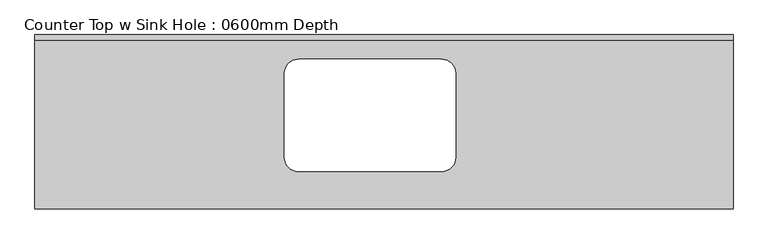
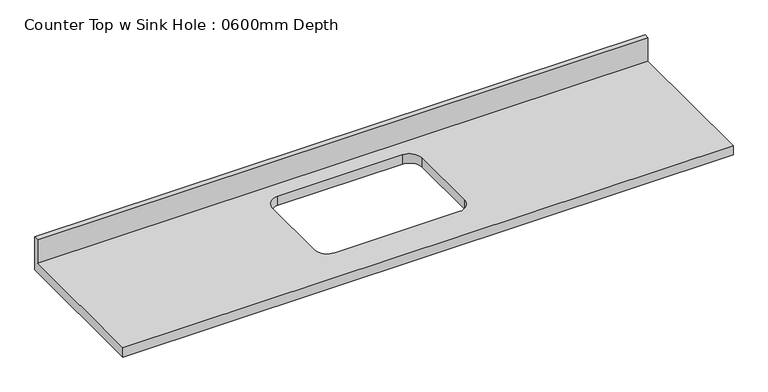
"""IFC4 building model written with IfcOpenShell, lengths in millimetres: furniture geometry, Counter Top w Sink Hole : 0600mm Depth."""

from ifc_helpers import new_model, si_unit, frame, origin, place, context, project, spatial, polyline, circle_curve, source, transform, mapped, element, save
from ifc_brep_helpers import plane_surface, revolved_surface, advanced_brep


def counter_top_w_sink_hole_0600mm_depth_f226a61d(model_context):
    return source(origin(), model_context, "Body", "AdvancedBrep", [
        advanced_brep(
        [(-1200.4622951, -624.68125, 900.1125), (1299.8502049, -624.68125, 900.1125), (1299.8502049, -19.05, 900.1125), (-1200.4622951, -19.05, 900.1125), (-255.8997951, -87.3125, 900.1125), (255.2752049, -87.3125, 900.1125), (306.0752049, -138.1125, 900.1125), (306.0752049, -439.7375, 900.1125), (255.2752049, -490.5375, 900.1125), (-255.8997951, -490.5375, 900.1125), (-306.6997951, -439.7375, 900.1125), (-306.6997951, -138.1125, 900.1125), (1299.8502049, 0.0, 860.425), (1299.8502049, -624.68125, 860.425), (-1200.4622951, -624.68125, 860.425), (-1200.4622951, 0.0, 860.425), (255.2752049, -87.3125, 860.425), (-255.8997951, -87.3125, 860.425), (-306.6997951, -138.1125, 860.425), (-306.6997951, -439.7375, 860.425), (-255.8997951, -490.5375, 860.425), (255.2752049, -490.5375, 860.425), (306.0752049, -439.7375, 860.425), (306.0752049, -138.1125, 860.425), (-1200.4622951, 0.0, 1001.7125), (1299.8502049, 0.0, 1001.7125), (-1200.4622951, -19.05, 1001.7125), (1299.8502049, -19.05, 1001.7125)],
        [
            (0, 1),
            (1, 2),
            (2, 3),
            (3, 0),
            (4, 5),
            (5, 6, circle_curve(frame((255.2752049, -138.1125, 900.1125), z_axis=(0.0, 0.0, -1.0), x_axis=(1.0, 0.0, 0.0)), 50.8)),
            (6, 7),
            (7, 8, circle_curve(frame((255.2752049, -439.7375, 900.1125), z_axis=(0.0, 0.0, -1.0), x_axis=(1.0, 0.0, 0.0)), 50.8)),
            (8, 9),
            (9, 10, circle_curve(frame((-255.8997951, -439.7375, 900.1125), z_axis=(0.0, 0.0, -1.0), x_axis=(1.0, 0.0, 0.0)), 50.8)),
            (10, 11),
            (11, 4, circle_curve(frame((-255.8997951, -138.1125, 900.1125), z_axis=(0.0, 0.0, -1.0), x_axis=(1.0, 0.0, 0.0)), 50.8)),
            (12, 13),
            (13, 14),
            (14, 15),
            (15, 12),
            (16, 17),
            (17, 18, circle_curve(frame((-255.8997951, -138.1125, 860.425), z_axis=(0.0, 0.0, 1.0), x_axis=(1.0, 0.0, 0.0)), 50.8)),
            (18, 19),
            (19, 20, circle_curve(frame((-255.8997951, -439.7375, 860.425), z_axis=(0.0, 0.0, 1.0), x_axis=(1.0, 0.0, 0.0)), 50.8)),
            (20, 21),
            (21, 22, circle_curve(frame((255.2752049, -439.7375, 860.425), z_axis=(0.0, 0.0, 1.0), x_axis=(1.0, 0.0, 0.0)), 50.8)),
            (22, 23),
            (23, 16, circle_curve(frame((255.2752049, -138.1125, 860.425), z_axis=(0.0, 0.0, 1.0), x_axis=(1.0, 0.0, 0.0)), 50.8)),
            (15, 24),
            (24, 25),
            (25, 12),
            (14, 0),
            (3, 26),
            (26, 24),
            (13, 1),
            (25, 27),
            (27, 2),
            (26, 27),
            (4, 17),
            (16, 5),
            (11, 18),
            (10, 19),
            (9, 20),
            (8, 21),
            (7, 22),
            (6, 23),
        ],
        [
            plane_surface(frame((-1200.4622951, 0.0, 900.1125), z_axis=(0.0, 0.0, 1.0), x_axis=(-1.0, 0.0, 0.0))),
            plane_surface(frame((-1200.4622951, 0.0, 860.425), z_axis=(0.0, 0.0, -1.0), x_axis=(1.0, 0.0, 0.0))),
            plane_surface(frame((1299.8502049, 0.0, 900.1125), z_axis=(0.0, 1.0, 0.0), x_axis=(0.0, 0.0, -1.0))),
            plane_surface(frame((-1200.4622951, 0.0, 900.1125), z_axis=(-1.0, 0.0, 0.0), x_axis=(0.0, 0.0, -1.0))),
            plane_surface(frame((-1200.4622951, -624.68125, 900.1125), z_axis=(0.0, -1.0, 0.0), x_axis=(0.0, 0.0, -1.0))),
            plane_surface(frame((1299.8502049, -624.68125, 900.1125), z_axis=(1.0, 0.0, 0.0), x_axis=(0.0, 0.0, -1.0))),
            plane_surface(frame((-1200.4622951, 0.0, 1001.7125), z_axis=(0.0, 0.0, 1.0), x_axis=(0.0, -1.0, 0.0))),
            plane_surface(frame((-1200.4622951, -19.05, 1001.7125), z_axis=(0.0, -1.0, 0.0), x_axis=(0.0, 0.0, -1.0))),
            plane_surface(frame((255.2752049, -87.3125, 900.1125), z_axis=(0.0, -1.0, 0.0), x_axis=(0.0, 0.0, -1.0))),
            revolved_surface(polyline([(-205.0997951, -138.1125, 900.1125), (-205.0997951, -138.1125, 860.425)]), (-255.8997951, -138.1125, 860.425), (0.0, 0.0, 1.0)),
            plane_surface(frame((-306.6997951, -138.1125, 900.1125), z_axis=(1.0, 0.0, 0.0), x_axis=(0.0, 0.0, -1.0))),
            revolved_surface(polyline([(-205.0997951, -439.7375, 900.1125), (-205.0997951, -439.7375, 860.425)]), (-255.8997951, -439.7375, 860.425), (0.0, 0.0, 1.0)),
            plane_surface(frame((-255.8997951, -490.5375, 900.1125), z_axis=(0.0, 1.0, 0.0), x_axis=(0.0, 0.0, -1.0))),
            revolved_surface(polyline([(306.0752049, -439.7375, 900.1125), (306.0752049, -439.7375, 860.425)]), (255.2752049, -439.7375, 860.425), (0.0, 0.0, 1.0)),
            plane_surface(frame((306.0752049, -439.7375, 900.1125), z_axis=(-1.0, 0.0, 0.0), x_axis=(0.0, 0.0, -1.0))),
            revolved_surface(polyline([(306.0752049, -138.1125, 900.1125), (306.0752049, -138.1125, 860.425)]), (255.2752049, -138.1125, 860.425), (0.0, 0.0, 1.0)),
        ],
        [
            (0, [[1, 2, 3, 4], [5, 6, 7, 8, 9, 10, 11, 12]]),
            (1, [[13, 14, 15, 16], [17, 18, 19, 20, 21, 22, 23, 24]]),
            (2, [[-16, 25, 26, 27]]),
            (3, [[-15, 28, -4, 29, 30, -25]]),
            (4, [[-1, -28, -14, 31]]),
            (5, [[-13, -27, 32, 33, -2, -31]]),
            (6, [[-30, 34, -32, -26]]),
            (7, [[-34, -29, -3, -33]]),
            (8, [[35, -17, 36, -5]]),
            (9, [[-35, -12, 37, -18]]),
            (10, [[-37, -11, 38, -19]]),
            (11, [[-38, -10, 39, -20]]),
            (12, [[-39, -9, 40, -21]]),
            (13, [[-40, -8, 41, -22]]),
            (14, [[-41, -7, 42, -23]]),
            (15, [[-36, -24, -42, -6]]),
        ],
    ),
    ])


if __name__ == "__main__":
    model = new_model("IFC4")
    model_context = context("Model", 3, world=origin())
    ifc_project = project(units=[si_unit("LENGTHUNIT", "METRE", prefix="MILLI")], contexts=[model_context])
    site = spatial("IfcSite", under=ifc_project)
    building = spatial("IfcBuilding", under=site)
    placement = place(None, origin())
    counter_top_w_sink_hole_0600mm_depth_shape = counter_top_w_sink_hole_0600mm_depth_f226a61d(model_context)
    element("IfcFurniture", 1, ObjectType="Counter Top w Sink Hole : 0600mm Depth", at=placement, inside=building, context=model_context, shape_type="MappedRepresentation", body=[
        mapped(counter_top_w_sink_hole_0600mm_depth_shape, transform((0.0, 0.0, 0.0), x_axis=(1.0, 0.0, 0.0), y_axis=(0.0, 1.0, 0.0), z_axis=(0.0, 0.0, 1.0))),
    ])
    save(model, "model.ifc")

# Revit data of these elements
# Type "Counter Top w Sink Hole : 0600mm Depth"
#   Assembly Code = "C1030400"
#   Counter Thickness = 0' - 1 9/16"
#   Depth [instance default] = 2' - 0 19/32"
#   Height = 2' - 11 7/16"
#   Length [instance default] = 8' - 2 7/16"
#   Sink Location [instance default] = 3' - 11 1/4"
#   Sink Location To Wall [instance default] = 0' - 3 15/16"
#   Sink Opening Depth [instance default] = 1' - 2 7/8"
#   Sink Opening Width [instance default] = 1' - 11 1/8"
#   Counter Top Material = none
#   Default Elevation = 0
# Element 1 (IfcFurniture, "Counter Top w Sink Hole : 0600mm Depth")
#   Materials on its faces: "Counter Top"
# Materials
#   "Counter Top": class "Wood", colour RGB 226 177 128, transparency 0
